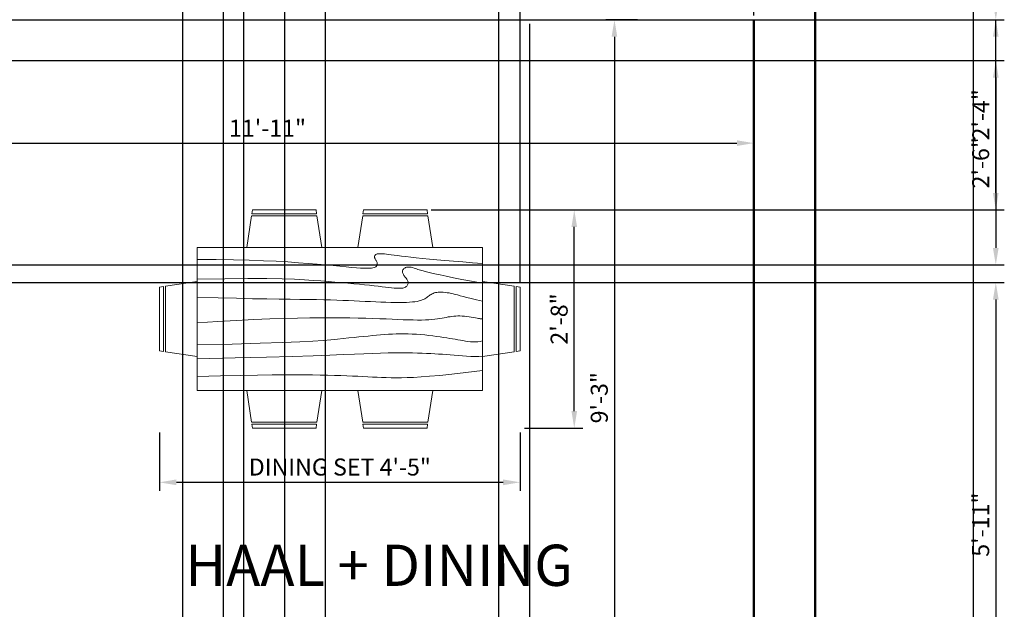
# Model space of a CAD drawing. Units: inches. Extents: x 1071 to 1348, y 2363 to 2916.
# Tile 3 of 4: x 1202 to 1347, y 2660 to 2746. Entities that reach past the tile are written whole.
import ezdxf

# ---------------------------------------------------------------- set-up
doc = ezdxf.new("R2010")
doc.units = ezdxf.units.IN
for name, color, linetype, lineweight in [('A-ANNO-DIMS', 2, 'Continuous', 18), ('A-AREA-IDEN', 7, 'Continuous', 25), ('A-FURN', 8, 'Continuous', 18), ('A-WALL', 7, 'Continuous', 50)]:
    doc.layers.add(name, color=color, linetype=linetype, lineweight=lineweight)
doc.styles.get("Standard").update_dxf_attribs({"font": 'arial.ttf'})
doc.dimstyles.new('ISO-25', dxfattribs={"dimtxt": 2.5, "dimasz": 2.5, "dimexe": 1.25, "dimexo": 0.625, "dimtad": 1, "dimdec": 0, "dimlunit": 3, "dimtxsty": 'Standard', "dimcen": 2.5, "dimadec": 0, "dimazin": 0, "dimtfac": 1, "dimtdec": 0, "dimtmove": 0, "dimatfit": 3, "dimfxl": 1, "dimarcsym": 0})

# ---------------------------------------------------------------- blocks, each defined once
blk = doc.blocks.new('Dining Set - 36 x 72 in.')
for p, q in [((-22, 27.5), (-22.1562, 26.50042)), ((-22, 27.5), (-6, 27.5)), ((-5.8437, 26.49966), (-6, 27.5)), ((6, 27.5), (5.8438, 26.50042)), ((6, 27.5), (22, 27.5)), ((22.1563, 26.49966), (22, 27.5)), ((-22.2343, 26.00059), (-23.4847, 17.99762)), ((-22.2304, 26), (-5.7608, 26)), ((-5.8416, 26.5), (-22.1534, 26.5)), ((-4.5152, 17.99762), (-5.7655, 25.99926)), ((5.7657, 26.00059), (4.5153, 17.99762)), ((5.7696, 26), (22.2392, 26)), ((22.1584, 26.5), (5.8466, 26.5)), ((23.4848, 17.99762), (22.2345, 25.99926)), ((36, 18), (-36, 18)), ((-36, 18), (-36, -18)), ((36, -18), (36, 18)), ((-45.5, 8), (-44.5004, 8.15617)), ((-45.5, 8), (-45.5, -8)), ((-44.5, -8.15843), (-44.5, 8.15338)), ((-44.0006, 8.23428), (-35.9976, 9.48474)), ((-44, 8.23041), (-44, -8.23915)), ((44.0006, 8.23428), (35.9976, 9.48474)), ((44, 8.23041), (44, -8.23915)), ((44.5, -8.15843), (44.5, 8.15338)), ((45.5, 8), (44.5005, 8.15617)), ((45.5, 8), (45.5, -8)), ((-44.4997, -8.15631), (-45.5, -8)), ((-35.9976, -9.48476), (-43.9993, -8.2345)), ((35.9976, -9.48476), (43.9993, -8.2345)), ((44.4997, -8.15631), (45.5, -8)), ((-36, -18), (36, -18)), ((-22.2343, -26.0006), (-23.4847, -17.99762)), ((-4.5152, -17.99762), (-5.7655, -25.99928)), ((5.7657, -26.0006), (4.5153, -17.99762)), ((23.4848, -17.99762), (22.2345, -25.99928)), ((-22.2304, -26), (-5.7608, -26)), ((-22, -27.5), (-22.1562, -26.50044)), ((-5.8416, -26.5), (-22.1534, -26.5)), ((-5.8437, -26.49967), (-6, -27.5)), ((5.7696, -26), (22.2392, -26)), ((6, -27.5), (5.8438, -26.50044)), ((22.1584, -26.5), (5.8466, -26.5)), ((22.1563, -26.49967), (22, -27.5)), ((-22, -27.5), (-6, -27.5)), ((6, -27.5), (22, -27.5))]:
    blk.add_line(p, q)
for points in [[(-36, 15), (-31.1772, 14.97754), (-26.8079, 14.91406), (-22.8538, 14.81543), (-19.276, 14.6875), (-16.0362, 14.53613), (-13.0957, 14.36718), (-10.4159, 14.18652), (-7.9583, 14), (-5.6904, 13.81315), (-3.6035, 13.63021), (-1.6954, 13.45508), (0.0365, 13.29166), (1.5945, 13.14388), (2.9811, 13.01562), (4.1988, 12.9108), (5.25, 12.83333), (6.1393, 12.78613), (6.8802, 12.76823), (7.4883, 12.77767), (7.9792, 12.8125), (8.3685, 12.87077), (8.6719, 12.95052), (8.9049, 13.0498), (9.0833, 13.16666), (9.2205, 13.29899), (9.3216, 13.44401), (9.3895, 13.59879), (9.4271, 13.76041), (9.4373, 13.92594), (9.4232, 14.09245), (9.3875, 14.257), (9.3333, 14.41666), (9.2638, 14.56917), (9.1836, 14.71484), (9.0975, 14.85465), (9.0104, 14.98958), (8.9272, 15.1206), (8.8529, 15.2487), (8.7922, 15.37483), (8.75, 15.5), (8.7305, 15.62467), (8.7344, 15.74739), (8.7617, 15.86621), (8.8125, 15.97916), (8.8867, 16.08431), (8.9844, 16.17968), (9.1055, 16.26334), (9.25, 16.33333), (9.4189, 16.38802), (9.6172, 16.42708), (9.8506, 16.45052), (10.125, 16.45833), (10.4463, 16.45052), (10.8203, 16.42708), (11.2529, 16.38802), (11.75, 16.33333), (12.3184, 16.26318), (12.9694, 16.17838), (13.7151, 16.07991), (14.5677, 15.96875), (15.5395, 15.84586), (16.6426, 15.71224), (17.8893, 15.56884), (19.2917, 15.41666), (20.859, 15.25667), (22.5879, 15.08984), (24.4721, 14.91715), (26.5052, 14.73958), (28.6809, 14.5581), (30.9929, 14.3737), (33.4347, 14.18733), (36, 14)], [(-36, 10), (-28.9766, 10.14274), (-23.1725, 10.20442), (-18.4241, 10.19775), (-14.5677, 10.13541), (-11.4399, 10.03011), (-8.877, 9.89453), (-6.7154, 9.74137), (-4.7917, 9.58333), (-2.9698, 9.43082), (-1.2246, 9.28515), (0.4415, 9.14534), (2.026, 9.01041), (3.5266, 8.87939), (4.9408, 8.7513), (6.266, 8.62516), (7.5, 8.5), (8.6411, 8.37549), (9.6914, 8.2539), (10.6538, 8.13818), (11.5312, 8.03125), (12.3267, 7.93603), (13.043, 7.85547), (13.6831, 7.79248), (14.25, 7.75), (14.7471, 7.7303), (15.1797, 7.73307), (15.5537, 7.75732), (15.875, 7.80208), (16.1494, 7.86637), (16.3828, 7.94922), (16.5811, 8.04964), (16.75, 8.16666), (16.8944, 8.29915), (17.0143, 8.44531), (17.1089, 8.60319), (17.1771, 8.77083), (17.218, 8.94629), (17.2305, 9.1276), (17.2137, 9.31282), (17.1667, 9.5), (17.0895, 9.6875), (16.987, 9.875), (16.8649, 10.0625), (16.7292, 10.25), (16.5856, 10.4375), (16.4401, 10.625), (16.2985, 10.8125), (16.1667, 11), (16.05, 11.18733), (15.9518, 11.3737), (15.8752, 11.5581), (15.8229, 11.73958), (15.798, 11.91715), (15.8034, 12.08984), (15.842, 12.25667), (15.9167, 12.41666), (16.0295, 12.56836), (16.1784, 12.70833), (16.3605, 12.83268), (16.5729, 12.9375), (16.8127, 13.01888), (17.0768, 13.07291), (17.3625, 13.0957), (17.6667, 13.08333), (17.9894, 13.03312), (18.3418, 12.94726), (18.7382, 12.82918), (19.1927, 12.68229), (19.7195, 12.51001), (20.3327, 12.31575), (21.0465, 12.10294), (21.875, 11.875), (22.8357, 11.63354), (23.959, 11.37304), (25.2786, 11.08618), (26.8282, 10.76562), (28.6414, 10.40405), (30.752, 9.99414), (33.1936, 9.52856), (36, 9)], [(-36, 5.5), (-30.7157, 5.3348), (-26.069, 5.20963), (-21.9946, 5.11767), (-18.4271, 5.05208), (-15.3009, 5.00602), (-12.5508, 4.97265), (-10.1112, 4.94515), (-7.9167, 4.91666), (-5.909, 4.88167), (-4.0586, 4.83984), (-2.3429, 4.79215), (-0.7396, 4.73958), (0.7739, 4.6831), (2.22, 4.6237), (3.6213, 4.56233), (5, 4.5), (6.373, 4.43782), (7.7344, 4.3776), (9.0723, 4.32129), (10.375, 4.27083), (11.6309, 4.22819), (12.8281, 4.19531), (13.9551, 4.17415), (15, 4.16666), (15.954, 4.17448), (16.819, 4.19791), (17.6001, 4.23698), (18.3021, 4.29166), (18.9299, 4.36198), (19.4883, 4.44791), (19.9823, 4.54948), (20.4167, 4.66666), (20.7969, 4.79899), (21.1302, 4.94401), (21.4245, 5.09879), (21.6875, 5.26041), (21.9271, 5.42594), (22.1511, 5.59245), (22.3672, 5.757), (22.5834, 5.91666), (22.8065, 6.06868), (23.0404, 6.21093), (23.2879, 6.34147), (23.5521, 6.45833), (23.8358, 6.55957), (24.142, 6.64323), (24.4735, 6.70735), (24.8334, 6.75), (25.2235, 6.76969), (25.642, 6.76692), (26.0858, 6.74267), (26.5521, 6.69791), (27.0379, 6.63362), (27.5404, 6.55078), (28.0565, 6.45036), (28.5834, 6.33333), (29.1242, 6.19987), (29.7071, 6.04687), (30.3661, 5.87044), (31.1354, 5.66666), (32.0493, 5.43164), (33.142, 5.16146), (34.4475, 4.85221), (36, 4.5)], [(-36, -1), (-30.7915, -0.6591), (-26.0195, -0.38216), (-21.6519, -0.16284), (-17.6563, 0.00521), (-14.0005, 0.12833), (-10.6523, 0.21289), (-7.5796, 0.26522), (-4.75, 0.29166), (-2.134, 0.29793), (0.2878, 0.28711), (2.5317, 0.26163), (4.6146, 0.22396), (6.5529, 0.17651), (8.3633, 0.12174), (10.0623, 0.06209), (11.6667, 0), (13.1899, -0.06201), (14.6341, -0.1211), (15.9982, -0.17432), (17.2813, -0.21875), (18.4823, -0.25147), (19.6003, -0.26953), (20.6343, -0.27002), (21.5834, -0.25), (22.4481, -0.20768), (23.2357, -0.14584), (23.9549, -0.06836), (24.6146, 0.02083), (25.2235, 0.11784), (25.7904, 0.21875), (26.3241, 0.31966), (26.8334, 0.41666), (27.3265, 0.50618), (27.8099, 0.58593), (28.2894, 0.65397), (28.7709, 0.70833), (29.2601, 0.74707), (29.763, 0.76823), (30.2855, 0.76985), (30.8334, 0.75), (31.4088, 0.70784), (31.9994, 0.64713), (32.589, 0.57275), (33.1615, 0.48958), (33.7008, 0.4025), (34.1908, 0.3164), (34.6153, 0.23616), (34.9584, 0.16666), (35.2099, 0.11165), (35.3848, 0.07031), (35.504, 0.04069), (35.5886, 0.02083), (35.6594, 0.00879), (35.7377, 0.0026), (35.8442, 0.00032), (36, 0)], [(-36, -6.5), (-27.1843, -6.31267), (-20.084, -6.1263), (-14.469, -5.9419), (-10.1094, -5.76042), (-6.7752, -5.58285), (-4.2363, -5.41016), (-2.2629, -5.24333), (-0.625, -5.08334), (0.8708, -4.93099), (2.2715, -4.78646), (3.5872, -4.64974), (4.8281, -4.52084), (6.0046, -4.39974), (7.127, -4.28646), (8.2053, -4.18099), (9.25, -4.08334), (10.2705, -3.99382), (11.2734, -3.91407), (12.2647, -3.84603), (13.25, -3.79167), (14.2354, -3.75293), (15.2266, -3.73177), (16.2295, -3.73015), (17.25, -3.75), (18.2912, -3.79248), (19.3451, -3.85547), (20.4009, -3.93604), (21.4479, -4.03125), (22.4754, -4.13819), (23.4727, -4.25391), (24.4289, -4.37549), (25.3334, -4.5), (26.1785, -4.62492), (26.9694, -4.74935), (27.7145, -4.87281), (28.4219, -4.99479), (29.1, -5.11483), (29.7572, -5.23242), (30.4016, -5.34709), (31.0417, -5.45834), (31.6837, -5.56437), (32.3262, -5.65821), (32.9658, -5.73153), (33.599, -5.77604), (34.2224, -5.78345), (34.8327, -5.74545), (35.4264, -5.65373), (36, -5.5)], [(-36, -10), (-26.4022, -9.81299), (-18.4675, -9.62891), (-11.9839, -9.45069), (-6.7396, -9.28125), (-2.5226, -9.12354), (0.8789, -8.98047), (3.6769, -8.85498), (6.0833, -8.75), (8.2767, -8.66765), (10.3021, -8.60677), (12.1712, -8.56543), (13.8958, -8.54167), (15.4876, -8.53353), (16.9583, -8.53907), (18.3197, -8.55632), (19.5834, -8.58334), (20.7616, -8.61841), (21.8685, -8.66081), (22.9188, -8.71004), (23.9271, -8.76563), (24.9081, -8.82707), (25.8763, -8.89388), (26.8465, -8.96558), (27.8334, -9.04167), (28.8474, -9.12118), (29.8828, -9.20117), (30.93, -9.27824), (31.9792, -9.34896), (33.0205, -9.40991), (34.0443, -9.45768), (35.0407, -9.48885), (36, -9.5)], [(-36, -14.5), (-30.0881, -14.33513), (-25.0332, -14.21224), (-20.7312, -14.12647), (-17.0781, -14.07292), (-13.97, -14.04671), (-11.3027, -14.04297), (-8.9724, -14.05681), (-6.875, -14.08334), (-4.9224, -14.11833), (-3.0905, -14.16016), (-1.3709, -14.20785), (0.2448, -14.26042), (1.7647, -14.3169), (3.1973, -14.3763), (4.5507, -14.43767), (5.8333, -14.5), (7.0554, -14.5621), (8.235, -14.62175), (9.3922, -14.67652), (10.5469, -14.72396), (11.7192, -14.76164), (12.929, -14.78711), (14.1965, -14.79794), (15.5417, -14.79167), (16.9933, -14.76424), (18.6152, -14.70508), (20.4804, -14.60197), (22.6615, -14.44271), (25.2312, -14.21509), (28.2624, -13.9069), (31.8277, -13.50594), (36, -13)]]:
    blk.add_lwpolyline(points)
blk = doc.blocks.new('*D13')
at = {"layer": 'A-ANNO-DIMS', "color": 0, "lineweight": -2, "transparency": 16777216}
for p, q in [((1293.16, 2746.25), (1288.53, 2746.25)), ((1289.78, 2743.75), (1289.78, 2637.75)), ((1290.91, 2635.25), (1288.53, 2635.25))]:
    blk.add_line(p, q, dxfattribs=at)
at = {"layer": 'A-ANNO-DIMS', "color": 0, "transparency": 16777216}
for points in [[(1289.36, 2743.75), (1290.19, 2743.75), (1289.78, 2746.25)], [(1289.36, 2637.75), (1290.19, 2637.75), (1289.78, 2635.25)]]:
    blk.add_solid(points, dxfattribs=at)
at = {"layer": 'Defpoints', "color": 0, "transparency": 16777216}
for p in [(1293.78, 2746.25), (1289.78, 2635.25), (1291.53, 2635.25)]:
    blk.add_point(p, dxfattribs=at)
at = {"layer": 'A-ANNO-DIMS', "color": 0, "transparency": 16777216, "insert": (1287.87, 2690.75), "char_height": 2.5, "attachment_point": 5, "rotation": 90}
blk.add_mtext('9\'-3"', dxfattribs=at)
blk = doc.blocks.new('*D14')
at = {"layer": 'A-ANNO-DIMS', "color": 0, "lineweight": -2, "transparency": 16777216}
for p, q in [((1167.28, 2710.88), (1167.28, 2729.38)), ((1169.78, 2728.13), (1307.78, 2728.13)), ((1310.28, 2710.88), (1310.28, 2729.38))]:
    blk.add_line(p, q, dxfattribs=at)
at = {"layer": 'A-ANNO-DIMS', "color": 0, "transparency": 16777216}
for points in [[(1169.78, 2728.55), (1169.78, 2727.72), (1167.28, 2728.13)], [(1307.78, 2728.55), (1307.78, 2727.72), (1310.28, 2728.13)]]:
    blk.add_solid(points, dxfattribs=at)
at = {"layer": 'Defpoints', "color": 0, "transparency": 16777216}
for p in [(1310.28, 2728.13), (1167.28, 2710.25), (1310.28, 2710.25)]:
    blk.add_point(p, dxfattribs=at)
at = {"layer": 'A-ANNO-DIMS', "color": 0, "transparency": 16777216, "insert": (1238.78, 2730.01), "char_height": 2.5, "attachment_point": 5}
blk.add_mtext('11\'-11"', dxfattribs=at)
blk = doc.blocks.new('*D21')
at = {"layer": 'A-ANNO-DIMS', "color": 0, "lineweight": -2, "transparency": 16777216}
for p, q in [((1319.91, 2884.25), (1343.77, 2884.25)), ((1342.52, 2881.75), (1342.52, 2393.75)), ((1319.91, 2391.25), (1343.77, 2391.25))]:
    blk.add_line(p, q, dxfattribs=at)
at = {"layer": 'A-ANNO-DIMS', "color": 0, "transparency": 16777216}
for points in [[(1342.11, 2881.75), (1342.94, 2881.75), (1342.52, 2884.25)], [(1342.11, 2393.75), (1342.94, 2393.75), (1342.52, 2391.25)]]:
    blk.add_solid(points, dxfattribs=at)
at = {"layer": 'Defpoints', "color": 0, "transparency": 16777216}
for p in [(1319.28, 2884.25), (1319.28, 2391.25), (1342.52, 2391.25)]:
    blk.add_point(p, dxfattribs=at)
at = {"layer": 'A-ANNO-DIMS', "color": 0, "transparency": 16777216, "insert": (1340.64, 2637.75), "char_height": 2.5, "attachment_point": 5, "rotation": 90}
blk.add_mtext('41\'-1"', dxfattribs=at)
blk = doc.blocks.new('*D39')
at = {"layer": 'A-ANNO-DIMS', "color": 0, "lineweight": -2, "transparency": 16777216}
for p, q in [((1222.89, 2685.66), (1222.89, 2677.08)), ((1275.92, 2685.66), (1275.92, 2677.08)), ((1225.39, 2678.33), (1273.42, 2678.33))]:
    blk.add_line(p, q, dxfattribs=at)
at = {"layer": 'A-ANNO-DIMS', "color": 0, "transparency": 16777216}
for points in [[(1225.39, 2678.75), (1225.39, 2677.91), (1222.89, 2678.33)], [(1273.42, 2678.75), (1273.42, 2677.91), (1275.92, 2678.33)]]:
    blk.add_solid(points, dxfattribs=at)
at = {"layer": 'Defpoints', "color": 0, "transparency": 16777216}
for p in [(1222.89, 2686.28), (1275.92, 2686.28), (1275.92, 2678.33)]:
    blk.add_point(p, dxfattribs=at)
at = {"layer": 'A-ANNO-DIMS', "color": 0, "transparency": 16777216, "insert": (1249.41, 2680.25), "char_height": 2.5, "attachment_point": 5}
blk.add_mtext('DINING SET 4\'-5"', dxfattribs=at)
blk = doc.blocks.new('*D40')
at = {"layer": 'A-ANNO-DIMS', "color": 0, "lineweight": -2, "transparency": 16777216}
for p, q in [((1276.55, 2718.33), (1285.12, 2718.33)), ((1283.87, 2688.78), (1283.87, 2715.83)), ((1276.55, 2686.28), (1285.12, 2686.28))]:
    blk.add_line(p, q, dxfattribs=at)
at = {"layer": 'A-ANNO-DIMS', "color": 0, "transparency": 16777216}
for points in [[(1283.46, 2715.83), (1284.29, 2715.83), (1283.87, 2718.33)], [(1283.46, 2688.78), (1284.29, 2688.78), (1283.87, 2686.28)]]:
    blk.add_solid(points, dxfattribs=at)
at = {"layer": 'Defpoints', "color": 0, "transparency": 16777216}
for p in [(1275.92, 2718.33), (1283.87, 2718.33), (1275.92, 2686.28)]:
    blk.add_point(p, dxfattribs=at)
at = {"layer": 'A-ANNO-DIMS', "color": 0, "transparency": 16777216, "insert": (1281.97, 2702.31), "char_height": 2.5, "attachment_point": 5, "rotation": 90}
blk.add_mtext('2\'-8"', dxfattribs=at)
blk = doc.blocks.new('*D48')
at = {"layer": 'A-ANNO-DIMS', "color": 0, "lineweight": -2, "transparency": 16777216}
for p, q in [((1184.28, 2745.63), (1184.28, 2363.45)), ((1226.28, 2745.63), (1226.28, 2363.45)), ((1186.78, 2364.7), (1223.78, 2364.7))]:
    blk.add_line(p, q, dxfattribs=at)
at = {"layer": 'A-ANNO-DIMS', "color": 0, "transparency": 16777216}
for points in [[(1186.78, 2365.12), (1186.78, 2364.29), (1184.28, 2364.7)], [(1223.78, 2365.12), (1223.78, 2364.29), (1226.28, 2364.7)]]:
    blk.add_solid(points, dxfattribs=at)
at = {"layer": 'Defpoints', "color": 0, "transparency": 16777216}
for p in [(1184.28, 2746.25), (1226.28, 2746.25), (1226.28, 2364.7)]:
    blk.add_point(p, dxfattribs=at)
at = {"layer": 'A-ANNO-DIMS', "color": 0, "transparency": 16777216, "insert": (1205.28, 2366.61), "char_height": 2.5, "attachment_point": 5}
blk.add_mtext('3\'-6"', dxfattribs=at)
blk = doc.blocks.new('*D49')
at = {"layer": 'A-ANNO-DIMS', "color": 0, "lineweight": -2, "transparency": 16777216}
for p, q in [((1247.28, 2745.63), (1247.28, 2363.45)), ((1277.28, 2745.63), (1277.28, 2363.45)), ((1249.78, 2364.7), (1274.78, 2364.7))]:
    blk.add_line(p, q, dxfattribs=at)
at = {"layer": 'A-ANNO-DIMS', "color": 0, "transparency": 16777216}
for points in [[(1249.78, 2365.12), (1249.78, 2364.29), (1247.28, 2364.7)], [(1274.78, 2365.12), (1274.78, 2364.29), (1277.28, 2364.7)]]:
    blk.add_solid(points, dxfattribs=at)
at = {"layer": 'Defpoints', "color": 0, "transparency": 16777216}
for p in [(1247.28, 2746.25), (1277.28, 2746.25), (1277.28, 2364.7)]:
    blk.add_point(p, dxfattribs=at)
at = {"layer": 'A-ANNO-DIMS', "color": 0, "transparency": 16777216, "insert": (1262.28, 2366.61), "char_height": 2.5, "attachment_point": 5}
blk.add_mtext('2\'-6"', dxfattribs=at)
blk = doc.blocks.new('*D50')
at = {"layer": 'A-ANNO-DIMS', "color": 0, "lineweight": -2, "transparency": 16777216}
for p, q in [((1169.91, 2740.25), (1347.08, 2740.25)), ((1345.83, 2737.75), (1345.83, 2712.75)), ((1169.91, 2710.25), (1347.08, 2710.25))]:
    blk.add_line(p, q, dxfattribs=at)
at = {"layer": 'A-ANNO-DIMS', "color": 0, "transparency": 16777216}
for points in [[(1345.41, 2737.75), (1346.25, 2737.75), (1345.83, 2740.25)], [(1345.41, 2712.75), (1346.25, 2712.75), (1345.83, 2710.25)]]:
    blk.add_solid(points, dxfattribs=at)
at = {"layer": 'Defpoints', "color": 0, "transparency": 16777216}
for p in [(1169.28, 2740.25), (1169.28, 2710.25), (1345.83, 2710.25)]:
    blk.add_point(p, dxfattribs=at)
at = {"layer": 'A-ANNO-DIMS', "color": 0, "transparency": 16777216, "insert": (1343.93, 2725.25), "char_height": 2.5, "attachment_point": 5, "rotation": 90}
blk.add_mtext('2\'-6"', dxfattribs=at)
blk = doc.blocks.new('*D52')
at = {"layer": 'A-ANNO-DIMS', "color": 0, "lineweight": -2, "transparency": 16777216}
for p, q in [((1345.83, 2748.75), (1345.83, 2759.15)), ((1160.91, 2746.25), (1347.08, 2746.25)), ((1345.83, 2740.25), (1345.83, 2746.25)), ((1169.91, 2740.25), (1347.08, 2740.25)), ((1345.83, 2737.75), (1345.83, 2735.25))]:
    blk.add_line(p, q, dxfattribs=at)
at = {"layer": 'A-ANNO-DIMS', "color": 0, "transparency": 16777216}
for points in [[(1345.41, 2748.75), (1346.25, 2748.75), (1345.83, 2746.25)], [(1345.41, 2737.75), (1346.25, 2737.75), (1345.83, 2740.25)]]:
    blk.add_solid(points, dxfattribs=at)
at = {"layer": 'Defpoints', "color": 0, "transparency": 16777216}
for p in [(1160.28, 2746.25), (1345.83, 2746.25), (1169.28, 2740.25)]:
    blk.add_point(p, dxfattribs=at)
at = {"layer": 'A-ANNO-DIMS', "color": 0, "transparency": 16777216, "insert": (1343.93, 2755.2), "char_height": 2.5, "attachment_point": 5, "rotation": 90}
blk.add_mtext('0\'-6"', dxfattribs=at)
blk = doc.blocks.new('*D53')
at = {"layer": 'A-ANNO-DIMS', "color": 0, "lineweight": -2, "transparency": 16777216}
for p, q in [((1226.28, 2754.63), (1226.28, 2363.45)), ((1232.28, 2754.63), (1232.28, 2363.45)), ((1223.78, 2364.7), (1221.28, 2364.7)), ((1226.28, 2364.7), (1232.28, 2364.7)), ((1234.78, 2364.7), (1245.18, 2364.7))]:
    blk.add_line(p, q, dxfattribs=at)
at = {"layer": 'A-ANNO-DIMS', "color": 0, "transparency": 16777216}
for points in [[(1223.78, 2365.12), (1223.78, 2364.29), (1226.28, 2364.7)], [(1234.78, 2365.12), (1234.78, 2364.29), (1232.28, 2364.7)]]:
    blk.add_solid(points, dxfattribs=at)
at = {"layer": 'Defpoints', "color": 0, "transparency": 16777216}
for p in [(1226.28, 2755.25), (1232.28, 2755.25), (1232.28, 2364.7)]:
    blk.add_point(p, dxfattribs=at)
at = {"layer": 'A-ANNO-DIMS', "color": 0, "transparency": 16777216, "insert": (1241.23, 2366.61), "char_height": 2.5, "attachment_point": 5}
blk.add_mtext('0\'-6"', dxfattribs=at)
blk = doc.blocks.new('*D54')
at = {"layer": 'A-ANNO-DIMS', "color": 0, "lineweight": -2, "transparency": 16777216}
for p, q in [((1241.28, 2754.63), (1241.28, 2363.45)), ((1247.28, 2754.63), (1247.28, 2363.45)), ((1238.78, 2364.7), (1236.28, 2364.7)), ((1241.28, 2364.7), (1247.28, 2364.7)), ((1249.78, 2364.7), (1260.18, 2364.7))]:
    blk.add_line(p, q, dxfattribs=at)
at = {"layer": 'A-ANNO-DIMS', "color": 0, "transparency": 16777216}
for points in [[(1238.78, 2365.12), (1238.78, 2364.29), (1241.28, 2364.7)], [(1249.78, 2365.12), (1249.78, 2364.29), (1247.28, 2364.7)]]:
    blk.add_solid(points, dxfattribs=at)
at = {"layer": 'Defpoints', "color": 0, "transparency": 16777216}
for p in [(1241.28, 2755.25), (1247.28, 2755.25), (1247.28, 2364.7)]:
    blk.add_point(p, dxfattribs=at)
at = {"layer": 'A-ANNO-DIMS', "color": 0, "transparency": 16777216, "insert": (1256.23, 2366.61), "char_height": 2.5, "attachment_point": 5}
blk.add_mtext('0\'-6"', dxfattribs=at)
blk = doc.blocks.new('*D56')
at = {"layer": 'A-ANNO-DIMS', "color": 0, "lineweight": -2, "transparency": 16777216}
for p, q in [((1235.28, 2497.88), (1235.28, 2912.05)), ((1272.78, 2497.88), (1272.78, 2912.05)), ((1237.78, 2910.8), (1270.28, 2910.8))]:
    blk.add_line(p, q, dxfattribs=at)
at = {"layer": 'A-ANNO-DIMS', "color": 0, "transparency": 16777216}
for points in [[(1237.78, 2911.22), (1237.78, 2910.39), (1235.28, 2910.8)], [(1270.28, 2911.22), (1270.28, 2910.39), (1272.78, 2910.8)]]:
    blk.add_solid(points, dxfattribs=at)
at = {"layer": 'Defpoints', "color": 0, "transparency": 16777216}
for p in [(1272.78, 2910.8), (1235.28, 2497.25), (1272.78, 2497.25)]:
    blk.add_point(p, dxfattribs=at)
at = {"layer": 'A-ANNO-DIMS', "color": 0, "transparency": 16777216, "insert": (1254.03, 2912.72), "char_height": 2.5, "attachment_point": 5}
blk.add_mtext('3\'-1 1/2"', dxfattribs=at)
blk = doc.blocks.new('*D66')
at = {"layer": 'A-ANNO-DIMS', "color": 0, "lineweight": -2, "transparency": 16777216}
for p, q in [((1193.46, 2707.65), (1347.08, 2707.65)), ((1345.83, 2705.15), (1345.83, 2639.07)), ((1216.75, 2636.57), (1347.08, 2636.57))]:
    blk.add_line(p, q, dxfattribs=at)
at = {"layer": 'A-ANNO-DIMS', "color": 0, "transparency": 16777216}
for points in [[(1345.41, 2705.15), (1346.25, 2705.15), (1345.83, 2707.65)], [(1345.41, 2639.07), (1346.25, 2639.07), (1345.83, 2636.57)]]:
    blk.add_solid(points, dxfattribs=at)
at = {"layer": 'Defpoints', "color": 0, "transparency": 16777216}
for p in [(1192.84, 2707.65), (1216.12, 2636.57), (1345.83, 2636.57)]:
    blk.add_point(p, dxfattribs=at)
at = {"layer": 'A-ANNO-DIMS', "color": 0, "transparency": 16777216, "insert": (1343.93, 2672.11), "char_height": 2.5, "attachment_point": 5, "rotation": 90}
blk.add_mtext('5\'-11"', dxfattribs=at)
blk = doc.blocks.new('*D67')
at = {"layer": 'A-ANNO-DIMS', "color": 0, "lineweight": -2, "transparency": 16777216}
for p, q in [((1275.92, 2707.6), (1275.92, 2912.05)), ((1310.28, 2746.88), (1310.28, 2912.05)), ((1278.42, 2910.8), (1307.78, 2910.8))]:
    blk.add_line(p, q, dxfattribs=at)
at = {"layer": 'A-ANNO-DIMS', "color": 0, "transparency": 16777216}
for points in [[(1278.42, 2911.22), (1278.42, 2910.39), (1275.92, 2910.8)], [(1307.78, 2911.22), (1307.78, 2910.39), (1310.28, 2910.8)]]:
    blk.add_solid(points, dxfattribs=at)
at = {"layer": 'Defpoints', "color": 0, "transparency": 16777216}
for p in [(1310.28, 2910.8), (1310.28, 2746.25), (1275.92, 2706.97)]:
    blk.add_point(p, dxfattribs=at)
at = {"layer": 'A-ANNO-DIMS', "color": 0, "transparency": 16777216, "insert": (1293.1, 2912.72), "char_height": 2.5, "attachment_point": 5}
blk.add_mtext('2\'-10 1/2"', dxfattribs=at)
blk = doc.blocks.new('*D68')
at = {"layer": 'A-ANNO-DIMS', "color": 0, "lineweight": -2, "transparency": 16777216}
for p, q in [((1277.91, 2746.25), (1347.08, 2746.25)), ((1345.83, 2720.83), (1345.83, 2743.75)), ((1262.85, 2718.33), (1347.08, 2718.33))]:
    blk.add_line(p, q, dxfattribs=at)
at = {"layer": 'A-ANNO-DIMS', "color": 0, "transparency": 16777216}
for points in [[(1345.41, 2743.75), (1346.25, 2743.75), (1345.83, 2746.25)], [(1345.41, 2720.83), (1346.25, 2720.83), (1345.83, 2718.33)]]:
    blk.add_solid(points, dxfattribs=at)
at = {"layer": 'Defpoints', "color": 0, "transparency": 16777216}
for p in [(1277.28, 2746.25), (1345.83, 2746.25), (1262.23, 2718.33)]:
    blk.add_point(p, dxfattribs=at)
at = {"layer": 'A-ANNO-DIMS', "color": 0, "transparency": 16777216, "insert": (1343.95, 2732.29), "char_height": 2.5, "attachment_point": 5, "rotation": 90}
blk.add_mtext('2\'-4"', dxfattribs=at)

msp = doc.modelspace()

# ---------------------------------------------------------------- linework, layer by layer
at = {"layer": 'A-WALL'}
for p, q in [((1319.28, 2884.25), (1319.28, 2391.25)), ((1310.28, 2746.25), (1310.28, 2635.25))]:
    msp.add_line(p, q, dxfattribs=at)

# ---------------------------------------------------------------- block references
at = {"layer": 'A-FURN', "xscale": 0.5827408066143699, "yscale": 0.5827408066143699, "zscale": 0.5827408066143699}
msp.add_blockref('Dining Set - 36 x 72 in.', (1249.41, 2702.31), dxfattribs=at)

# ---------------------------------------------------------------- texts
at = {"layer": 'A-AREA-IDEN'}
msp.add_text('HAAL + DINING', height=6.0552, dxfattribs=at).set_placement((1226.69, 2663.12))

# ---------------------------------------------------------------- dimensions: what is measured, and where the dimension line sits
at = {"layer": 'A-ANNO-DIMS'}
for base, p1, p2, override, picture, middle in [((1272.78, 2910.8), (1235.28, 2497.25), (1272.78, 2497.25), {"dimdec": 1, "dimlfac": 1, "dimrnd": 0, "dimzin": 1, "dimdsep": 46, "dimlunit": 4, "dimfrac": 2}, '*D56', (1254.03, 2912.72)), ((1310.28, 2910.8), (1275.92, 2706.97), (1310.28, 2746.25), {"dimdec": 1, "dimlfac": 1, "dimrnd": 0, "dimzin": 1, "dimdsep": 46, "dimlunit": 4, "dimfrac": 2}, '*D67', (1293.1, 2912.72)), ((1232.28, 2364.7), (1226.28, 2755.25), (1232.28, 2755.25), {"dimdec": 1, "dimlfac": 1, "dimrnd": 0, "dimzin": 1, "dimdsep": 46, "dimlunit": 4, "dimfrac": 2}, '*D53', (1241.23, 2366.61)), ((1247.28, 2364.7), (1241.28, 2755.25), (1247.28, 2755.25), {"dimdec": 1, "dimlfac": 1, "dimrnd": 0, "dimzin": 1, "dimdsep": 46, "dimlunit": 4, "dimfrac": 2}, '*D54', (1256.23, 2366.61)), ((1226.28, 2364.7), (1184.28, 2746.25), (1226.28, 2746.25), {"dimdec": 1, "dimlfac": 1, "dimrnd": 0, "dimzin": 1, "dimdsep": 46, "dimlunit": 4, "dimfrac": 2}, '*D48', (1205.28, 2366.61)), ((1277.28, 2364.7), (1247.28, 2746.25), (1277.28, 2746.25), {"dimdec": 1, "dimlfac": 1, "dimrnd": 0, "dimzin": 1, "dimdsep": 46, "dimlunit": 4, "dimfrac": 2}, '*D49', (1262.28, 2366.61)), ((1310.28, 2728.13), (1167.28, 2710.25), (1310.28, 2710.25), {"dimclrd": 0, "dimclre": 0, "dimclrt": 0}, '*D14', (1238.78, 2730.01))]:
    dim = msp.add_linear_dim(base=base, p1=p1, p2=p2, dimstyle='ISO-25', override=override, dxfattribs=at)
    dim.commit()
    dim.dimension.update_dxf_attribs({"geometry": picture, "text_midpoint": middle})
for base, p1, p2, override, picture, middle in [((1342.52, 2391.25), (1319.28, 2884.25), (1319.28, 2391.25), {"dimclrd": 0, "dimclre": 0, "dimclrt": 0}, '*D21', (1340.64, 2637.75)), ((1345.83, 2746.25), (1169.28, 2740.25), (1160.28, 2746.25), {"dimdec": 1, "dimlfac": 1, "dimrnd": 0, "dimzin": 1, "dimdsep": 46, "dimlunit": 4, "dimfrac": 2}, '*D52', (1343.93, 2755.2)), ((1345.83, 2746.25), (1262.23, 2718.33), (1277.28, 2746.25), {"dimdec": 1, "dimlfac": 1, "dimrnd": 0, "dimzin": 1, "dimdsep": 46, "dimlunit": 4, "dimfrac": 2}, '*D68', (1343.95, 2732.29)), ((1289.78, 2635.25), (1293.78, 2746.25), (1291.53, 2635.25), {"dimclrd": 0, "dimclre": 0, "dimclrt": 0}, '*D13', (1287.87, 2690.75)), ((1345.83, 2710.25), (1169.28, 2740.25), (1169.28, 2710.25), {"dimdec": 1, "dimlfac": 1, "dimrnd": 0, "dimzin": 1, "dimdsep": 46, "dimlunit": 4, "dimfrac": 2}, '*D50', (1343.93, 2725.25)), ((1283.8749, 2718.3338), (1275.9205, 2686.283), (1275.9205, 2718.3338), {"dimdec": 1, "dimlfac": 1, "dimrnd": 0, "dimzin": 1, "dimdsep": 46, "dimlunit": 4, "dimfrac": 2}, '*D40', (1281.9734, 2702.3084)), ((1345.83, 2636.57), (1192.84, 2707.65), (1216.12, 2636.57), {"dimdec": 1, "dimlfac": 1, "dimrnd": 0, "dimzin": 1, "dimdsep": 46, "dimlunit": 4, "dimfrac": 2}, '*D66', (1343.93, 2672.11))]:
    dim = msp.add_linear_dim(base=base, p1=p1, p2=p2, angle=90, dimstyle='ISO-25', override=override, dxfattribs=at)
    dim.commit()
    dim.dimension.update_dxf_attribs({"geometry": picture, "text_midpoint": middle})
dim = msp.add_linear_dim(base=(1275.92, 2678.33), p1=(1222.89, 2686.28), p2=(1275.92, 2686.28), text='DINING SET <>', dimstyle='ISO-25', override={"dimdec": 1, "dimlfac": 1, "dimrnd": 0, "dimzin": 1, "dimdsep": 46, "dimlunit": 4, "dimfrac": 2}, dxfattribs=at)
dim.commit()
dim.dimension.update_dxf_attribs({"geometry": '*D39', "text_midpoint": (1249.41, 2680.25)})

doc.saveas('drawing.dxf')
